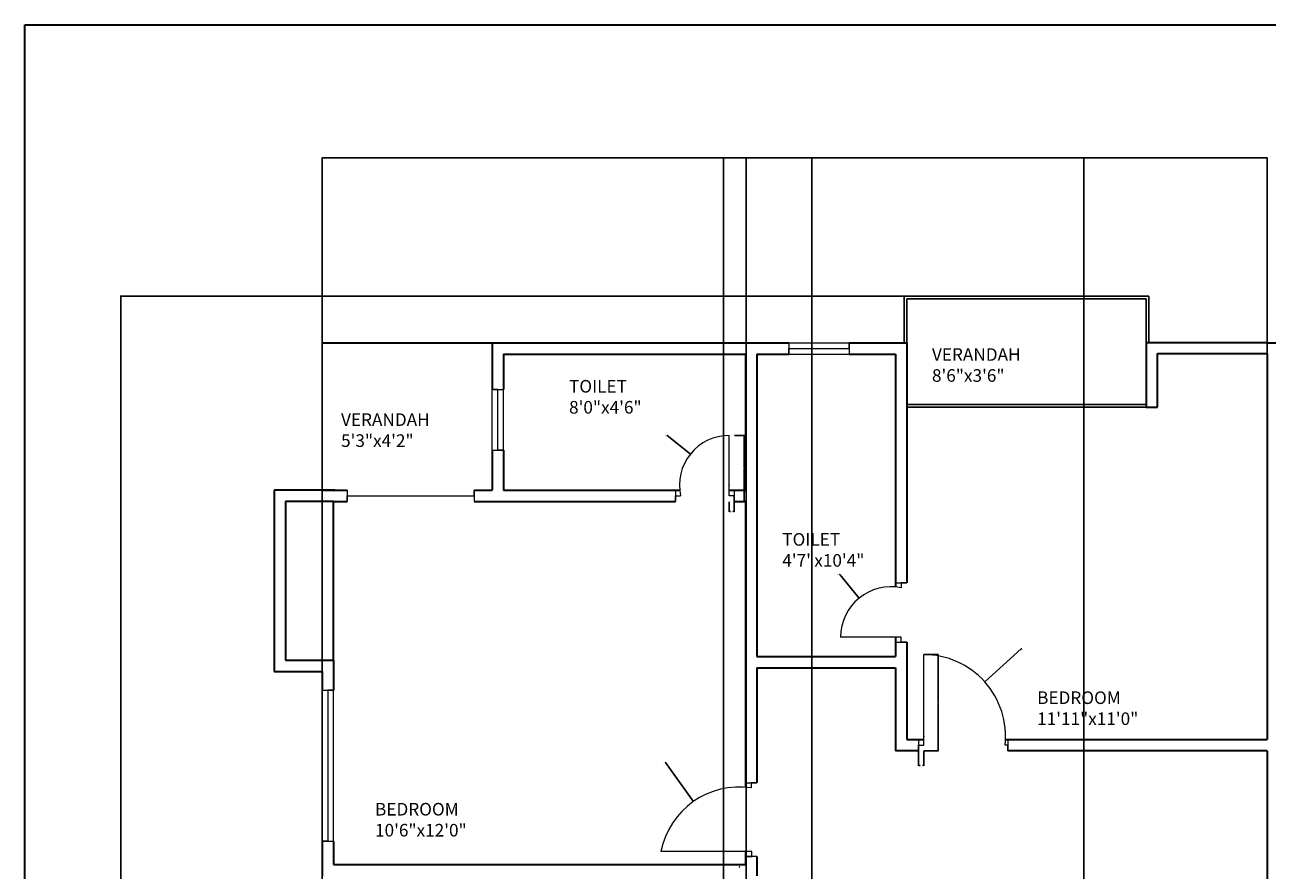
# Model space of a CAD drawing. Units: inches. Extents: x 2154 to 3131, y 1384 to 2688.
# Tile 3 of 5: x 2154 to 2647, y 2353 to 2688. Entities that reach past the tile are written whole.
import ezdxf

# ---------------------------------------------------------------- set-up
doc = ezdxf.new("R2010")
doc.units = ezdxf.units.IN
for name, color, linetype, lineweight in [('A-ANNO-DIMS', 2, 'Continuous', 18), ('A-ANNO-TTLB', 7, 'Continuous', 35), ('A-AREA-IDEN', 7, 'Continuous', 18), ('A-DOOR', 31, 'Continuous', 18), ('A-FLOR-BALC', 130, 'Continuous', 25), ('A-GLAZ', 130, 'Continuous', 18), ('A-WALL', 7, 'Continuous', 35)]:
    doc.layers.add(name, color=color, linetype=linetype, lineweight=lineweight)
doc.styles.get("Standard").update_dxf_attribs({"font": 'arial.ttf'})
doc.dimstyles.get("Standard").update_dxf_attribs({"dimtxt": 0.18, "dimasz": 0.18, "dimexe": 0.18, "dimexo": 0.0625, "dimgap": 0.09, "dimtad": 0, "dimtih": 1, "dimtoh": 1, "dimdec": 4, "dimzin": 0, "dimdsep": 46, "dimtxsty": 'Standard', "dimcen": 0.09, "dimadec": 0, "dimazin": 0, "dimtfac": 1, "dimtdec": 4, "dimtofl": 0, "dimtmove": 0, "dimatfit": 3, "dimfxl": 1, "dimtolj": 1, "dimtzin": 0, "dimarcsym": 0})

# ---------------------------------------------------------------- blocks, each defined once
blk = doc.blocks.new('DOOR-LEAF-24-JAMB-A')
for p, q in [((0, 2.25), (0, 26.25)), ((2, 2.25), (0, 2.25)), ((2, 4.5), (2, 0)), ((2, 0), (2, 2.25))]:
    blk.add_line(p, q)
blk = doc.blocks.new('DOOR-LEAF-36-JAMB-A')
for p, q in [((2, 2.25), (2, 38.25)), ((0, 4.5), (0, 0)), ((0, 0), (0, 2.25)), ((0, 2.25), (2, 2.25))]:
    blk.add_line(p, q)
blk = doc.blocks.new('WIN-24-FRAME-A')
for p, q in [((0, 4.5), (0, 0)), ((0, 4.5), (24, 4.5)), ((0, 0), (0, 2.25)), ((0, 2.25), (24, 2.25)), ((0, 0), (24, 0)), ((24, 2.25), (24, 4.5)), ((24, 4.5), (24, 0))]:
    blk.add_line(p, q)
blk = doc.blocks.new('WIN-60')
for p, q in [((2.25, 60), (0, 60)), ((0, 60), (4.5, 60)), ((0, 60), (0, 0)), ((2.25, 0), (2.25, 60)), ((4.5, 60), (4.5, 0)), ((0, 0), (4.5, 0)), ((4.5, 0), (2.25, 0))]:
    blk.add_line(p, q)
blk = doc.blocks.new('*D8')
at = {"layer": 'A-ANNO-DIMS', "color": 0, "lineweight": -2, "transparency": 16777216}
for p, q in [((2435.74, 2525.43), (2439.8, 2525.43)), ((2439.62, 2525.25), (2439.62, 2512.48)), ((2439.62, 2499.36), (2439.62, 2512.12)), ((2435.74, 2499.18), (2439.8, 2499.18))]:
    blk.add_line(p, q, dxfattribs=at)
at = {"layer": 'A-ANNO-DIMS', "color": 0, "transparency": 16777216}
for points in [[(2439.59, 2525.25), (2439.65, 2525.25), (2439.62, 2525.43)], [(2439.59, 2499.36), (2439.65, 2499.36), (2439.62, 2499.18)]]:
    blk.add_solid(points, dxfattribs=at)
at = {"layer": 'Defpoints', "color": 0, "transparency": 16777216}
for p in [(2435.68, 2525.43), (2439.62, 2525.43), (2435.68, 2499.18)]:
    blk.add_point(p, dxfattribs=at)
at = {"layer": 'A-ANNO-DIMS', "color": 0, "transparency": 16777216, "insert": (2439.62, 2512.3), "char_height": 0.18, "attachment_point": 5}
blk.add_mtext('\\A1;D1 26 TYP.', dxfattribs=at)
blk = doc.blocks.new('*D9')
at = {"layer": 'A-ANNO-DIMS', "color": 0, "lineweight": -2, "transparency": 16777216}
for p, q in [((2433.68, 2499.11), (2433.68, 2495.06)), ((2433.86, 2495.24), (2434.22, 2495.24)), ((2435.5, 2495.24), (2435.14, 2495.24)), ((2435.68, 2499.11), (2435.68, 2495.06))]:
    blk.add_line(p, q, dxfattribs=at)
at = {"layer": 'A-ANNO-DIMS', "color": 0, "transparency": 16777216}
for points in [[(2433.86, 2495.27), (2433.86, 2495.21), (2433.68, 2495.24)], [(2435.5, 2495.27), (2435.5, 2495.21), (2435.68, 2495.24)]]:
    blk.add_solid(points, dxfattribs=at)
at = {"layer": 'Defpoints', "color": 0, "transparency": 16777216}
for p in [(2433.68, 2499.18), (2435.68, 2499.18), (2435.68, 2495.24)]:
    blk.add_point(p, dxfattribs=at)
at = {"layer": 'A-ANNO-DIMS', "color": 0, "transparency": 16777216, "insert": (2434.68, 2495.24), "char_height": 0.18, "attachment_point": 5}
blk.add_mtext('\\A1;2 TYP.', dxfattribs=at)
blk = doc.blocks.new('*D12')
at = {"layer": 'A-ANNO-DIMS', "color": 0, "lineweight": -2, "transparency": 16777216}
for p, q in [((2510.94, 2438.43), (2516.79, 2438.43)), ((2516.61, 2438.25), (2516.61, 2419.48)), ((2516.61, 2400.36), (2516.61, 2419.12)), ((2510.94, 2400.18), (2516.79, 2400.18))]:
    blk.add_line(p, q, dxfattribs=at)
at = {"layer": 'A-ANNO-DIMS', "color": 0, "transparency": 16777216}
for points in [[(2516.58, 2438.25), (2516.64, 2438.25), (2516.61, 2438.43)], [(2516.58, 2400.36), (2516.64, 2400.36), (2516.61, 2400.18)]]:
    blk.add_solid(points, dxfattribs=at)
at = {"layer": 'Defpoints', "color": 0, "transparency": 16777216}
for p in [(2510.87, 2438.43), (2516.61, 2438.43), (2510.87, 2400.18)]:
    blk.add_point(p, dxfattribs=at)
at = {"layer": 'A-ANNO-DIMS', "color": 0, "transparency": 16777216, "insert": (2516.61, 2419.3), "char_height": 0.18, "attachment_point": 5}
blk.add_mtext('\\A1;D3 38 TYP.', dxfattribs=at)
blk = doc.blocks.new('*D13')
at = {"layer": 'A-ANNO-DIMS', "color": 0, "lineweight": -2, "transparency": 16777216}
for p, q in [((2508.87, 2400.11), (2508.87, 2394.26)), ((2510.87, 2400.11), (2510.87, 2394.26)), ((2509.05, 2394.44), (2509.41, 2394.44)), ((2510.69, 2394.44), (2510.33, 2394.44))]:
    blk.add_line(p, q, dxfattribs=at)
at = {"layer": 'A-ANNO-DIMS', "color": 0, "transparency": 16777216}
for points in [[(2509.05, 2394.47), (2509.05, 2394.41), (2508.87, 2394.44)], [(2510.69, 2394.47), (2510.69, 2394.41), (2510.87, 2394.44)]]:
    blk.add_solid(points, dxfattribs=at)
at = {"layer": 'Defpoints', "color": 0, "transparency": 16777216}
for p in [(2508.87, 2400.18), (2510.87, 2400.18), (2510.87, 2394.44)]:
    blk.add_point(p, dxfattribs=at)
at = {"layer": 'A-ANNO-DIMS', "color": 0, "transparency": 16777216, "insert": (2509.87, 2394.44), "char_height": 0.18, "attachment_point": 5}
blk.add_mtext('\\A1;2 TYP.', dxfattribs=at)
blk = doc.blocks.new('*D23')
at = {"layer": 'A-ANNO-DIMS', "color": 0, "lineweight": -2, "transparency": 16777216}
for p, q in [((2504.09, 2580.68), (2192.08, 2580.68)), ((2192.26, 2580.5), (2192.26, 2091.11)), ((2192.26, 1601.36), (2192.26, 2090.74)), ((2504.09, 1601.18), (2192.08, 1601.18))]:
    blk.add_line(p, q, dxfattribs=at)
at = {"layer": 'A-ANNO-DIMS', "color": 0, "transparency": 16777216}
for points in [[(2192.23, 2580.5), (2192.29, 2580.5), (2192.26, 2580.68)], [(2192.23, 1601.36), (2192.29, 1601.36), (2192.26, 1601.18)]]:
    blk.add_solid(points, dxfattribs=at)
at = {"layer": 'Defpoints', "color": 0, "transparency": 16777216}
for p in [(2192.26, 2580.68), (2504.16, 2580.68), (2504.16, 1601.18)]:
    blk.add_point(p, dxfattribs=at)
at = {"layer": 'A-ANNO-DIMS', "color": 0, "transparency": 16777216, "insert": (2192.26, 2090.93), "char_height": 0.18, "attachment_point": 5}
blk.add_mtext('\\A1;979.5', dxfattribs=at)
blk = doc.blocks.new('*D24')
at = {"layer": 'A-ANNO-DIMS', "color": 0, "lineweight": -2, "transparency": 16777216}
for p, q in [((2272.16, 2562.24), (2272.16, 2635.76)), ((2272.34, 2635.58), (2459.37, 2635.58)), ((2646.98, 2635.58), (2459.95, 2635.58)), ((2647.16, 2557.97), (2647.16, 2635.76))]:
    blk.add_line(p, q, dxfattribs=at)
at = {"layer": 'A-ANNO-DIMS', "color": 0, "transparency": 16777216}
for points in [[(2272.34, 2635.61), (2272.34, 2635.55), (2272.16, 2635.58)], [(2646.98, 2635.61), (2646.98, 2635.55), (2647.16, 2635.58)]]:
    blk.add_solid(points, dxfattribs=at)
at = {"layer": 'Defpoints', "color": 0, "transparency": 16777216}
for p in [(2647.16, 2635.58), (2272.16, 2562.18), (2647.16, 2557.91)]:
    blk.add_point(p, dxfattribs=at)
at = {"layer": 'A-ANNO-DIMS', "color": 0, "transparency": 16777216, "insert": (2459.66, 2635.58), "char_height": 0.18, "attachment_point": 5}
blk.add_mtext('\\A1;375', dxfattribs=at)
blk = doc.blocks.new('*D26')
at = {"layer": 'A-ANNO-DIMS', "color": 0, "lineweight": -2, "transparency": 16777216}
for p, q in [((2272.16, 2041.74), (2272.16, 2635.76)), ((2272.34, 2635.58), (2351.32, 2635.58)), ((2431.22, 2635.58), (2352.24, 2635.58)), ((2431.4, 2041.74), (2431.4, 2635.76))]:
    blk.add_line(p, q, dxfattribs=at)
at = {"layer": 'A-ANNO-DIMS', "color": 0, "transparency": 16777216}
for points in [[(2272.34, 2635.61), (2272.34, 2635.55), (2272.16, 2635.58)], [(2431.22, 2635.61), (2431.22, 2635.55), (2431.4, 2635.58)]]:
    blk.add_solid(points, dxfattribs=at)
at = {"layer": 'Defpoints', "color": 0, "transparency": 16777216}
for p in [(2431.4, 2635.58), (2272.16, 2041.68), (2431.4, 2041.68)]:
    blk.add_point(p, dxfattribs=at)
at = {"layer": 'A-ANNO-DIMS', "color": 0, "transparency": 16777216, "insert": (2351.78, 2635.58), "char_height": 0.18, "attachment_point": 5}
blk.add_mtext('\\A1;159.25', dxfattribs=at)
blk = doc.blocks.new('*D28')
at = {"layer": 'A-ANNO-DIMS', "color": 0, "lineweight": -2, "transparency": 16777216}
for p, q in [((2466.46, 2137.74), (2466.46, 2635.76)), ((2466.64, 2635.58), (2520.18, 2635.58)), ((2574.28, 2635.58), (2520.74, 2635.58)), ((2574.46, 2137.74), (2574.46, 2635.76))]:
    blk.add_line(p, q, dxfattribs=at)
at = {"layer": 'A-ANNO-DIMS', "color": 0, "transparency": 16777216}
for points in [[(2466.64, 2635.61), (2466.64, 2635.55), (2466.46, 2635.58)], [(2574.28, 2635.61), (2574.28, 2635.55), (2574.46, 2635.58)]]:
    blk.add_solid(points, dxfattribs=at)
at = {"layer": 'Defpoints', "color": 0, "transparency": 16777216}
for p in [(2574.46, 2635.58), (2466.46, 2137.68), (2574.46, 2137.68)]:
    blk.add_point(p, dxfattribs=at)
at = {"layer": 'A-ANNO-DIMS', "color": 0, "transparency": 16777216, "insert": (2520.46, 2635.58), "char_height": 0.18, "attachment_point": 5}
blk.add_mtext('\\A1;108', dxfattribs=at)
blk = doc.blocks.new('*D29')
at = {"layer": 'A-ANNO-DIMS', "color": 0, "lineweight": -2, "transparency": 16777216}
for p, q in [((2440.4, 2137.74), (2440.4, 2635.76)), ((2440.58, 2635.58), (2453.04, 2635.58)), ((2466.28, 2635.58), (2453.83, 2635.58)), ((2466.46, 2137.74), (2466.46, 2635.76))]:
    blk.add_line(p, q, dxfattribs=at)
at = {"layer": 'A-ANNO-DIMS', "color": 0, "transparency": 16777216}
for points in [[(2440.58, 2635.61), (2440.58, 2635.55), (2440.4, 2635.58)], [(2466.28, 2635.61), (2466.28, 2635.55), (2466.46, 2635.58)]]:
    blk.add_solid(points, dxfattribs=at)
at = {"layer": 'Defpoints', "color": 0, "transparency": 16777216}
for p in [(2466.46, 2635.58), (2440.4, 2137.68), (2466.46, 2137.68)]:
    blk.add_point(p, dxfattribs=at)
at = {"layer": 'A-ANNO-DIMS', "color": 0, "transparency": 16777216, "insert": (2453.43, 2635.58), "char_height": 0.18, "attachment_point": 5}
blk.add_mtext('\\A1;26.06', dxfattribs=at)
blk = doc.blocks.new('*D36')
at = {"layer": 'A-ANNO-DIMS', "color": 0, "lineweight": -2, "transparency": 16777216}
for p, q in [((2549.58, 2440.67), (2535.2, 2427.76)), ((2549.76, 2440.67), (2549.58, 2440.67)), ((2510.78, 2405.91), (2510.96, 2405.91)), ((2510.87, 2405.82), (2510.87, 2406))]:
    blk.add_line(p, q, dxfattribs=at)
at = {"layer": 'A-ANNO-DIMS', "color": 0, "transparency": 16777216}
blk.add_solid([(2535.18, 2427.78), (2535.22, 2427.73), (2535.06, 2427.64)], dxfattribs=at)
at = {"layer": 'Defpoints', "color": 0, "transparency": 16777216}
for p in [(2535.06, 2427.64), (2510.87, 2405.91)]:
    blk.add_point(p, dxfattribs=at)
at = {"layer": 'A-ANNO-DIMS', "color": 0, "transparency": 16777216, "insert": (2550.22, 2440.67), "char_height": 0.18, "attachment_point": 5}
blk.add_mtext('\\A1;R32.51', dxfattribs=at)
blk = doc.blocks.new('*D38')
at = {"layer": 'A-ANNO-DIMS', "color": 0, "lineweight": -2, "transparency": 16777216}
for p, q in [((2408.28, 2395.61), (2408.46, 2395.61)), ((2408.46, 2395.61), (2419.35, 2380.21)), ((2437.67, 2354.15), (2437.85, 2354.15)), ((2437.76, 2354.06), (2437.76, 2354.24))]:
    blk.add_line(p, q, dxfattribs=at)
at = {"layer": 'A-ANNO-DIMS', "color": 0, "transparency": 16777216}
blk.add_solid([(2419.37, 2380.23), (2419.32, 2380.19), (2419.45, 2380.06)], dxfattribs=at)
at = {"layer": 'Defpoints', "color": 0, "transparency": 16777216}
for p in [(2419.45, 2380.06), (2437.76, 2354.15)]:
    blk.add_point(p, dxfattribs=at)
at = {"layer": 'A-ANNO-DIMS', "color": 0, "transparency": 16777216, "insert": (2407.8, 2395.61), "char_height": 0.18, "attachment_point": 5}
blk.add_mtext('\\A1;R31.73', dxfattribs=at)
blk = doc.blocks.new('*D55')
at = {"layer": 'A-ANNO-DIMS', "color": 0, "lineweight": -2, "transparency": 16777216}
for p, q in [((2477.47, 2470.16), (2477.65, 2470.16)), ((2477.65, 2470.16), (2485.14, 2461)), ((2497.83, 2445.36), (2498.01, 2445.36)), ((2497.92, 2445.27), (2497.92, 2445.45))]:
    blk.add_line(p, q, dxfattribs=at)
at = {"layer": 'A-ANNO-DIMS', "color": 0, "transparency": 16777216}
blk.add_solid([(2485.16, 2461.02), (2485.12, 2460.98), (2485.26, 2460.86)], dxfattribs=at)
at = {"layer": 'Defpoints', "color": 0, "transparency": 16777216}
for p in [(2485.26, 2460.86), (2497.92, 2445.36)]:
    blk.add_point(p, dxfattribs=at)
at = {"layer": 'A-ANNO-DIMS', "color": 0, "transparency": 16777216, "insert": (2476.92, 2470.16), "char_height": 0.18, "attachment_point": 5}
blk.add_mtext('\\A1;R20.016', dxfattribs=at)
blk = doc.blocks.new('*D56')
at = {"layer": 'A-ANNO-DIMS', "color": 0, "lineweight": -2, "transparency": 16777216}
for p, q in [((2408.88, 2525.45), (2409.06, 2525.45)), ((2409.06, 2525.45), (2418.15, 2518.16)), ((2433.59, 2505.7), (2433.77, 2505.7)), ((2433.68, 2505.61), (2433.68, 2505.79))]:
    blk.add_line(p, q, dxfattribs=at)
at = {"layer": 'A-ANNO-DIMS', "color": 0, "transparency": 16777216}
blk.add_solid([(2418.17, 2518.18), (2418.13, 2518.14), (2418.29, 2518.05)], dxfattribs=at)
at = {"layer": 'Defpoints', "color": 0, "transparency": 16777216}
for p in [(2418.29, 2518.05), (2433.68, 2505.7)]:
    blk.add_point(p, dxfattribs=at)
at = {"layer": 'A-ANNO-DIMS', "color": 0, "transparency": 16777216, "insert": (2408.33, 2525.45), "char_height": 0.18, "attachment_point": 5}
blk.add_mtext('\\A1;R19.728', dxfattribs=at)

msp = doc.modelspace()

# ---------------------------------------------------------------- linework, layer by layer
at = {"layer": 'A-ANNO-TTLB'}
msp.add_lwpolyline([(2154.1953, 2688.4009), (3131.1627, 2688.4009), (3131.1627, 1383.7377), (2154.1953, 1383.7377)], close=True, dxfattribs=at)
at = {"layer": 'A-DOOR'}
for p, q in [((2412.4197, 2503.6767), (2412.4197, 2503.6767)), ((2412.4197, 2503.6767), (2412.4197, 2503.6767)), ((2412.4197, 2503.6767), (2412.4197, 2499.1767)), ((2412.4197, 2499.1767), (2412.4197, 2501.4267)), ((2412.4197, 2501.4267), (2414.4197, 2501.4267)), ((2499.656, 2466.9787), (2504.156, 2466.9787)), ((2504.156, 2466.9787), (2501.906, 2466.9787)), ((2501.906, 2466.9787), (2501.906, 2464.9787)), ((2544.1968, 2402.4267), (2543.1968, 2402.4267)), ((2544.1968, 2404.6767), (2544.1968, 2400.1767)), ((2544.1968, 2400.1767), (2544.1968, 2402.4267)), ((2440.156, 2387.5355), (2444.656, 2387.5355)), ((2444.656, 2387.5355), (2442.406, 2387.5355)), ((2442.406, 2387.5355), (2442.406, 2385.5355)), ((2442.6216, 2360.253), (2406.6216, 2360.253)), ((2440.5872, 2358.253), (2440.156, 2358.253)), ((2440.156, 2358.253), (2442.6216, 2358.253)), ((2444.656, 2358.253), (2440.5872, 2358.253)), ((2442.6216, 2358.253), (2442.6216, 2360.253)), ((2442.6216, 2358.253), (2442.6216, 2358.253))]:
    msp.add_line(p, q, dxfattribs=at)
for centre, radius, start, end in [((2433.6791, 2505.6991), 19.7276, 90, 192.507651), ((2497.9224, 2445.3627), 20.0164, 78.520535, 180), ((2510.8726, 2405.9148), 32.5119, 353.840985, 90), ((2437.7601, 2354.1457), 31.7318, 81.581039, 168.903107)]:
    msp.add_arc(centre, radius, start, end, dxfattribs=at)
at = {"layer": 'A-FLOR-BALC'}
for p, q in [((2504.156, 2580.6767), (2503.156, 2580.6767)), ((2503.156, 2580.6767), (2503.156, 2562.1767)), ((2600.156, 2580.6767), (2504.156, 2580.6767)), ((2504.156, 2579.6767), (2599.156, 2579.6767)), ((2504.156, 2562.1767), (2504.156, 2579.6767)), ((2599.156, 2562.1767), (2599.156, 2579.6767)), ((2600.156, 2579.6767), (2600.156, 2580.6767)), ((2600.156, 2579.6767), (2600.156, 2562.1767)), ((2272.156, 2562.1767), (2272.156, 2503.6767)), ((2599.156, 2537.6767), (2504.156, 2537.6767)), ((2504.156, 2536.6767), (2599.156, 2536.6767)), ((2272.156, 2355.1767), (2272.156, 2354.1767))]:
    msp.add_line(p, q, dxfattribs=at)
at = {"layer": 'A-GLAZ'}
for p, q in [((2282.1432, 2503.6767), (2282.1432, 2499.1767)), ((2282.1432, 2499.1767), (2282.1432, 2501.4267)), ((2282.1432, 2501.4267), (2332.4845, 2501.4267)), ((2332.4845, 2501.4267), (2332.4845, 2503.6767)), ((2332.4845, 2503.6767), (2332.4845, 2503.6767)), ((2332.4845, 2503.6767), (2332.4845, 2499.1767)), ((2332.4845, 2501.4267), (2332.4845, 2501.4267))]:
    msp.add_line(p, q, dxfattribs=at)
at = {"layer": 'A-WALL'}
for p, q in [((2272.156, 2562.1767), (2457.3, 2562.1767)), ((2339.656, 2562.1767), (2339.656, 2543.629)), ((2481.3, 2562.1767), (2504.156, 2562.1767)), ((2504.156, 2562.1767), (2504.156, 2466.9787)), ((2647.156, 2562.1767), (2599.156, 2562.1767)), ((2599.156, 2562.1767), (2599.156, 2536.6767)), ((2647.156, 2562.1767), (2699.656, 2562.1767)), ((2344.156, 2557.6767), (2440.156, 2557.6767)), ((2344.156, 2557.6767), (2344.156, 2543.629)), ((2440.156, 2557.6767), (2440.156, 2503.6767)), ((2444.656, 2557.6767), (2444.656, 2437.6767)), ((2444.656, 2557.6767), (2457.3, 2557.6767)), ((2481.3, 2557.6767), (2499.656, 2557.6767)), ((2499.656, 2557.6767), (2499.656, 2465.3039)), ((2603.656, 2536.6767), (2603.656, 2557.9062)), ((2603.656, 2557.9062), (2647.156, 2557.9062)), ((2647.156, 2557.9062), (2647.156, 2404.6767)), ((2504.156, 2536.6767), (2504.156, 2466.9787)), ((2599.156, 2536.6767), (2600.156, 2536.6767)), ((2600.156, 2536.6767), (2602.156, 2536.6767)), ((2602.156, 2536.6767), (2603.656, 2536.6767)), ((2339.656, 2519.629), (2339.656, 2503.6767)), ((2344.156, 2519.629), (2344.156, 2503.6767)), ((2277.1496, 2503.6767), (2253.1496, 2503.6767)), ((2253.1496, 2503.6767), (2253.1496, 2455.6767)), ((2272.156, 2503.6767), (2282.1432, 2503.6767)), ((2332.4845, 2503.6767), (2339.656, 2503.6767)), ((2344.156, 2503.6767), (2414.0554, 2503.6767)), ((2433.6791, 2503.6767), (2440.156, 2503.6767)), ((2276.656, 2499.1767), (2257.6496, 2499.1767)), ((2257.6496, 2499.1767), (2257.6496, 2436.1767)), ((2276.656, 2499.1767), (2282.1432, 2499.1767)), ((2276.656, 2436.1767), (2276.656, 2499.1767)), ((2332.4845, 2499.1767), (2412.4197, 2499.1767)), ((2435.6791, 2499.1767), (2440.156, 2499.1767)), ((2440.156, 2499.1767), (2440.156, 2385.7869)), ((2253.1496, 2455.6767), (2253.1496, 2431.6767)), ((2499.656, 2445.3627), (2499.656, 2437.6767)), ((2504.156, 2443.3627), (2504.156, 2404.6767)), ((2504.156, 2443.3627), (2504.156, 2404.6767)), ((2257.6496, 2436.1767), (2276.656, 2436.1767)), ((2276.656, 2436.1767), (2276.656, 2424.3207)), ((2444.656, 2437.6767), (2499.656, 2437.6767)), ((2253.1496, 2431.6767), (2272.156, 2431.6767)), ((2272.156, 2431.6767), (2272.156, 2424.3207)), ((2444.656, 2433.1767), (2499.656, 2433.1767)), ((2444.656, 2433.1767), (2444.656, 2387.5355)), ((2499.656, 2433.1767), (2499.656, 2400.1767)), ((2504.156, 2404.6767), (2510.8726, 2404.6767)), ((2543.3609, 2404.6767), (2647.156, 2404.6767)), ((2508.8726, 2400.1767), (2499.656, 2400.1767)), ((2647.156, 2400.1767), (2544.1968, 2400.1767)), ((2647.156, 2400.1767), (2647.156, 2142.1767)), ((2272.156, 2364.3207), (2272.156, 2350.6767)), ((2276.656, 2364.3207), (2276.656, 2355.1767)), ((2440.156, 2360.253), (2440.156, 2355.1767)), ((2444.656, 2358.253), (2444.656, 2350.6767)), ((2276.656, 2355.1767), (2440.156, 2355.1767))]:
    msp.add_line(p, q, dxfattribs=at)

# ---------------------------------------------------------------- block references
at = {"layer": 'A-DOOR'}
for name, p in [('DOOR-LEAF-24-JAMB-A', (2433.6791, 2499.1767)), ('DOOR-LEAF-36-JAMB-A', (2508.8726, 2400.1767))]:
    msp.add_blockref(name, p, dxfattribs=at)
at = {"layer": 'A-DOOR', "extrusion": (0, 0, -1), "zscale": -1, "rotation": 270.0000000000001}
msp.add_blockref('DOOR-LEAF-24-JAMB-A', (-2504.156, 2445.3627), dxfattribs=at)
at = {"layer": 'A-GLAZ'}
msp.add_blockref('WIN-24-FRAME-A', (2457.3, 2557.6767), dxfattribs=at)
at = {"layer": 'A-GLAZ', "rotation": 90.00000000000627}
msp.add_blockref('WIN-24-FRAME-A', (2344.156, 2519.629), dxfattribs=at)
at = {"layer": 'A-GLAZ', "extrusion": (0, 0, -1), "zscale": -1, "rotation": 180}
msp.add_blockref('WIN-60', (-2272.156, 2424.3207), dxfattribs=at)

# ---------------------------------------------------------------- texts
at = {"layer": 'A-AREA-IDEN', "char_height": 5, "attachment_point": 1}
for s, width, insert in [('VERANDAH\\P8\'6"x3\'6"', 127.045563, (2514.1491, 2560.0443)), ('TOILET\\P8\'0"x4\'6"', 134.008072, (2370.1479, 2547.4302)), ('VERANDAH\\P5\'3"x4\'2"', 154.005541, (2279.6735, 2534.1913)), ('TOILET\\P4\'7"x10\'4"', 119.997994, (2454.7531, 2486.6536)), ('BEDROOM\\P11\'11"x11\'0"', 123.994984, (2555.8836, 2423.8179)), ('BEDROOM\\P10\'6"x12\'0"', 214.937604, (2293.1524, 2379.5597))]:
    msp.add_mtext_dynamic_manual_height_columns(s, width=width, gutter_width=12.5, heights=[0], dxfattribs=dict(at, insert=insert))

# ---------------------------------------------------------------- dimensions: what is measured, and where the dimension line sits
at = {"layer": 'A-ANNO-DIMS'}
for base, p1, p2, override, picture, middle in [((2647.156, 2635.5767), (2272.156, 2562.1767), (2647.156, 2557.9062), {"dimdec": 0, "dimlfac": 1, "dimrnd": 0, "dimzin": 0, "dimdsep": 46, "dimlunit": 2}, '*D24', (2459.656, 2635.5767)), ((2431.4046, 2635.5767), (2272.156, 2041.6767), (2431.4046, 2041.6767), {"dimdec": 2, "dimlfac": 1, "dimrnd": 0, "dimzin": 0, "dimdsep": 46, "dimlunit": 2}, '*D26', (2351.7803, 2635.5767)), ((2466.4638, 2635.5767), (2440.4046, 2137.6767), (2466.4638, 2137.6767), {"dimdec": 2, "dimlfac": 1, "dimrnd": 0, "dimzin": 0, "dimdsep": 46, "dimlunit": 2}, '*D29', (2453.4342, 2635.5767)), ((2574.4638, 2635.5767), (2466.4638, 2137.6767), (2574.4638, 2137.6767), {"dimdec": 0, "dimlfac": 1, "dimrnd": 0, "dimzin": 0, "dimdsep": 46, "dimlunit": 2}, '*D28', (2520.4638, 2635.5767))]:
    dim = msp.add_linear_dim(base=base, p1=p1, p2=p2, dimstyle='Standard', override=override, dxfattribs=at)
    dim.commit()
    dim.dimension.update_dxf_attribs({"geometry": picture, "text_midpoint": middle})
dim = msp.add_linear_dim(base=(2192.256, 2580.6767), p1=(2504.156, 1601.1767), p2=(2504.156, 2580.6767), angle=90, dimstyle='Standard', override={"dimdec": 1, "dimlfac": 1, "dimrnd": 0, "dimzin": 0, "dimdsep": 46, "dimlunit": 2}, dxfattribs=at)
dim.commit()
dim.dimension.update_dxf_attribs({"geometry": '*D23', "text_midpoint": (2192.256, 2090.9267)})
for center, mpoint, override, picture, middle in [((2433.6791, 2505.6991), (2418.293, 2518.046), {"dimdec": 3, "dimlfac": 1, "dimrnd": 0, "dimzin": 0, "dimdsep": 46, "dimlunit": 2}, '*D56', (2408.3314, 2525.4542)), ((2497.9224, 2445.3627), (2485.2551, 2460.8609), {"dimdec": 3, "dimlfac": 1, "dimrnd": 0, "dimzin": 0, "dimdsep": 46, "dimlunit": 2}, '*D55', (2476.925, 2470.1598)), ((2510.8726, 2405.9148), (2535.0639, 2427.6359), {"dimdec": 2, "dimlfac": 1, "dimrnd": 0, "dimzin": 0, "dimdsep": 46, "dimlunit": 2}, '*D36', (2550.2211, 2440.6685)), ((2437.7601, 2354.1457), (2419.4501, 2380.0619), {"dimdec": 2, "dimlfac": 1, "dimrnd": 0, "dimzin": 0, "dimdsep": 46, "dimlunit": 2}, '*D38', (2407.8042, 2395.6116))]:
    dim = msp.add_radius_dim(center=center, mpoint=mpoint, dimstyle='Standard', override=override, dxfattribs=at)
    dim.commit()
    dim.dimension.update_dxf_attribs({"geometry": picture, "text_midpoint": middle, "dimtype": 164})
for base, p1, p2, text, picture, middle in [((2439.6166, 2525.4267), (2435.6791, 2499.1767), (2435.6791, 2525.4267), 'D1 <> TYP.', '*D8', (2439.6166, 2512.3017)), ((2516.6101, 2438.4267), (2510.8726, 2400.1767), (2510.8726, 2438.4267), 'D3 <> TYP.', '*D12', (2516.6101, 2419.3017))]:
    dim = msp.add_linear_dim(base=base, p1=p1, p2=p2, angle=90, text=text, dimstyle='Standard', override={"dimdec": 0, "dimlfac": 1, "dimrnd": 0, "dimzin": 0, "dimdsep": 46, "dimlunit": 2}, dxfattribs=at)
    dim.commit()
    dim.dimension.update_dxf_attribs({"geometry": picture, "text_midpoint": middle})
for base, p1, p2, picture, middle in [((2435.6791, 2495.2392), (2433.6791, 2499.1767), (2435.6791, 2499.1767), '*D9', (2434.6791, 2495.2392)), ((2510.8726, 2394.4392), (2508.8726, 2400.1767), (2510.8726, 2400.1767), '*D13', (2509.8726, 2394.4392))]:
    dim = msp.add_linear_dim(base=base, p1=p1, p2=p2, text='<> TYP.', dimstyle='Standard', override={"dimdec": 0, "dimlfac": 1, "dimrnd": 0, "dimzin": 0, "dimdsep": 46, "dimlunit": 2}, dxfattribs=at)
    dim.commit()
    dim.dimension.update_dxf_attribs({"geometry": picture, "text_midpoint": middle})

doc.saveas('drawing.dxf')
